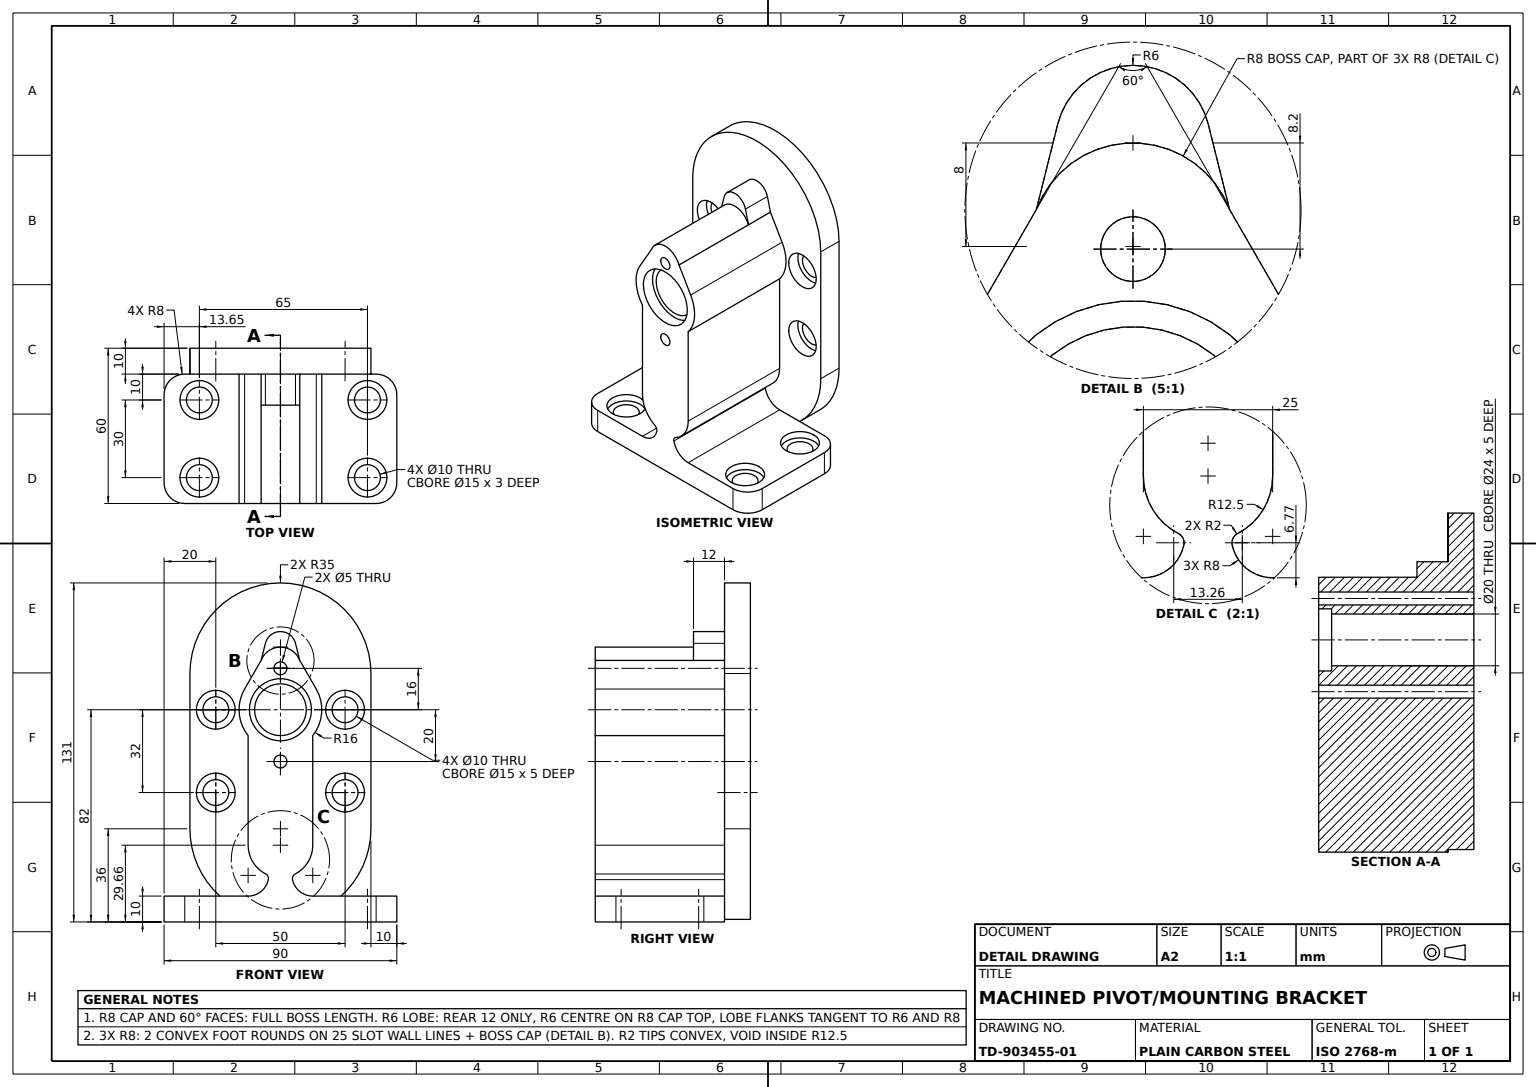
from build123d import *

# Parameters (mm, degrees)
FLANGE_PLATE_SKETCH_R     = 5
FLANGE_PLATE_DEPTH        = 10
FLANGE_START              = -5
FLANGE_RECESS_SKETCH_R    = 7.5
FLANGE_RECESS_SKETCH_R_2  = 5
FLANGE_RECESS_5MM_DEPTH   = 5
BRACKET_BODY_SKETCH_R     = 2.5
BRACKET_BODY_DEPTH        = 50
THROUGH_START             = -50
THROUGH_BORE_SKETCH_R     = 10
THROUGH_BORE_DEPTH        = 50
BORE_COUNTERBORE_SKETCH_R = 12
BORE_COUNTERBORE_24_DEPTH = 5
BODY_POCKET_SKETCH_R      = 5
BODY_POCKET_20MM_DEPTH    = 20
POCKET_STEP_SKETCH_R      = 7.5
POCKET_STEP_3MM_DEPTH     = 3
BODY_BOSS_12MM_DEPTH      = 12
BODY_FILLET_R8_A_R        = 8
BODY_FILLET_R8_B_R        = 8
BODY_SLOT_SKETCH_R        = 2.5
BODY_SLOT_CUT_DEPTH       = 112.126054551


with BuildPart() as part:
    # Flange Plate Sketch → Flange Plate (new body)
    with BuildSketch(Plane.XY):
        with BuildLine():
            Line((-35, -46), (-35, 14))
            ThreePointArc((-35, 14), (0, 49), (35, 14))
            Line((35, 14), (35, -46))
            ThreePointArc((35, -46), (0, -81), (-35, -46))
        make_face()
        with Locations((-25, 0)):
            Circle(FLANGE_PLATE_SKETCH_R, mode=Mode.SUBTRACT)
        with Locations((25, 0)):
            Circle(FLANGE_PLATE_SKETCH_R, mode=Mode.SUBTRACT)
        with Locations((-25, -32)):
            Circle(FLANGE_PLATE_SKETCH_R, mode=Mode.SUBTRACT)
        with Locations((25, -32)):
            Circle(FLANGE_PLATE_SKETCH_R, mode=Mode.SUBTRACT)
    extrude(amount=FLANGE_PLATE_DEPTH)

    # Flange Recess Sketch → Flange Recess 5mm (cut)
    # profile 1 of 4: a face of its own
    with BuildSketch(Plane.XY.offset(10).offset(FLANGE_START)):
        with Locations((-25, 0)):
            Circle(FLANGE_RECESS_SKETCH_R)
        with Locations((-25, 0)):
            Circle(FLANGE_RECESS_SKETCH_R_2, mode=Mode.SUBTRACT)
    # profile 2 of 4: a face of its own
    with BuildSketch(Plane.XY.offset(10).offset(FLANGE_START)):
        with Locations((25, 0)):
            Circle(FLANGE_RECESS_SKETCH_R)
        with Locations((25, 0)):
            Circle(FLANGE_RECESS_SKETCH_R_2, mode=Mode.SUBTRACT)
    # profile 3 of 4: a face of its own
    with BuildSketch(Plane.XY.offset(10).offset(FLANGE_START)):
        with Locations((25, -32)):
            Circle(FLANGE_RECESS_SKETCH_R)
        with Locations((25, -32)):
            Circle(FLANGE_RECESS_SKETCH_R_2, mode=Mode.SUBTRACT)
    # profile 4 of 4: a face of its own
    with BuildSketch(Plane.XY.offset(10).offset(FLANGE_START)):
        with Locations((-25, -32)):
            Circle(FLANGE_RECESS_SKETCH_R)
        with Locations((-25, -32)):
            Circle(FLANGE_RECESS_SKETCH_R_2, mode=Mode.SUBTRACT)
    extrude(amount=FLANGE_RECESS_5MM_DEPTH, mode=Mode.SUBTRACT)

    # Bracket Body Sketch → Bracket Body (add)
    # profile 1 of 2: a face of its own
    with BuildSketch(Plane.XY.offset(10)):
        with BuildLine():
            Line((-12.5, -72), (-23.430749028, -72))
            ThreePointArc((-23.430749028, -72), (0, -81), (23.430749028, -72))
            Line((23.430749028, -72), (12.5, -72))
            ThreePointArc((12.5, -72), (7.458524391, -70.211563707), (4.67113827, -65.645880922))
            ThreePointArc((4.67113827, -65.645880922), (4.822624016, -64.374561693), (5.714098019, -63.455608694))
            ThreePointArc((5.714098019, -63.455608694), (10.669494488, -58.85053718), (12.5, -52.33809621))
            Line((12.5, -52.33809621), (12.5, -9.987492178))
            ThreePointArc((12.5, -9.987492178), (15.954701786, -1.203117164), (13.856406461, 8))
            Line((13.856406461, 8), (7.473378872, 19.05572809))
            ThreePointArc((7.473378872, 19.05572809), (0, 24.201151372), (-7.473378872, 19.05572809))
            Line((-7.473378872, 19.05572809), (-13.856406461, 8))
            ThreePointArc((-13.856406461, 8), (-15.954701786, -1.203117164), (-12.5, -9.987492178))
            Line((-12.5, -9.987492178), (-12.5, -52.33809621))
            ThreePointArc((-12.5, -52.33809621), (-10.669494488, -58.85053718), (-5.714098019, -63.455608694))
            ThreePointArc((-5.714098019, -63.455608694), (-4.822624016, -64.374561693), (-4.67113827, -65.645880922))
            ThreePointArc((-4.67113827, -65.645880922), (-7.458524391, -70.211563707), (-12.5, -72))
        make_face()
        with Locations((0, -20)):
            Circle(BRACKET_BODY_SKETCH_R, mode=Mode.SUBTRACT)
        with BuildLine():
            ThreePointArc((0, -10), (-7.071067812, 7.071067812), (10, 0))
            ThreePointArc((10, 0), (7.071067812, -7.071067812), (0, -10))
        make_face(mode=Mode.SUBTRACT)
        with Locations((0, 16)):
            Circle(BRACKET_BODY_SKETCH_R, mode=Mode.SUBTRACT)
    # profile 2 of 2: a face of its own
    with BuildSketch(Plane.XY.offset(10)):
        with BuildLine():
            Line((-45, -72), (-45, -82))
            Line((-45, -82), (45, -82))
            Line((45, -82), (45, -72))
            Line((45, -72), (23.430749028, -72))
            ThreePointArc((23.430749028, -72), (0, -81), (-23.430749028, -72))
            Line((-23.430749028, -72), (-45, -72))
        make_face()
    extrude(amount=BRACKET_BODY_DEPTH)

    # Through Bore Sketch → Through Bore (cut)
    with BuildSketch(Plane.XY.offset(10).offset(THROUGH_START)):
        with Locations(Location((0, 0, 0), (0, 0, 180))):
            Circle(THROUGH_BORE_SKETCH_R)
    extrude(amount=THROUGH_BORE_DEPTH, mode=Mode.SUBTRACT)

    # Bore Counterbore Sketch → Bore Counterbore Ø24 (cut)
    with BuildSketch(Plane.XY.offset(60)):
        Circle(BORE_COUNTERBORE_SKETCH_R)
    extrude(amount=-BORE_COUNTERBORE_24_DEPTH, mode=Mode.SUBTRACT)

    # Body Pocket Sketch → Body Pocket 20mm (cut)
    with BuildSketch(Plane(origin=(0, -72, 0), x_dir=(1, 0, 0), z_dir=(0, 1, 0))):
        with Locations(Location((-31.350256263, -20, 0), (0, 0, 270))):
            Circle(BODY_POCKET_SKETCH_R)
        with Locations(Location((-31.350256263, -50, 0), (0, 0, 270))):
            Circle(BODY_POCKET_SKETCH_R)
        with Locations(Location((33.649743737, -20, 0), (0, 0, 270))):
            Circle(BODY_POCKET_SKETCH_R)
        with Locations(Location((33.649743737, -50, 0), (0, 0, 270))):
            Circle(BODY_POCKET_SKETCH_R)
    extrude(amount=-BODY_POCKET_20MM_DEPTH, mode=Mode.SUBTRACT)

    # Pocket Step Sketch → Pocket Step 3mm (cut)
    with BuildSketch(Plane(origin=(0, -72, 0), x_dir=(1, 0, 0), z_dir=(0, 1, 0))):
        with Locations(Location((-31.350256263, -20, 0), (0, 0, 270))):
            Circle(POCKET_STEP_SKETCH_R)
        with Locations(Location((-31.350256263, -50, 0), (0, 0, 270))):
            Circle(POCKET_STEP_SKETCH_R)
        with Locations(Location((33.649743737, -20, 0), (0, 0, 270))):
            Circle(POCKET_STEP_SKETCH_R)
        with Locations(Location((33.649743737, -50, 0), (0, 0, 270))):
            Circle(POCKET_STEP_SKETCH_R)
    extrude(amount=-POCKET_STEP_3MM_DEPTH, mode=Mode.SUBTRACT)

    # Body Boss Sketch → Body Boss 12mm (add)
    with BuildSketch(Plane.XY.offset(10)):
        with BuildLine():
            Line((7.473378872, 19.05572809), (5.820364134, 25.658327183))
            ThreePointArc((5.820364134, 25.658327183), (0, 30.201151372), (-5.820364134, 25.658327183))
            Line((-5.820364134, 25.658327183), (-7.473378872, 19.05572809))
            ThreePointArc((-7.473378872, 19.05572809), (0, 24.201151372), (7.473378872, 19.05572809))
        make_face()
    extrude(amount=BODY_BOSS_12MM_DEPTH)

    # Body Fillet R8 A
    body_fillet_r8_a_edges = [part.edges().sort_by_distance(p)[0] for p in [
        (-45, -77, 60),
        (45, -77, 60),
    ]]
    fillet(body_fillet_r8_a_edges, radius=BODY_FILLET_R8_A_R)

    # Body Fillet R8 B
    body_fillet_r8_b_edges = [part.edges().sort_by_distance(p)[0] for p in [
        (-45, -77, 10),
        (45, -77, 10),
    ]]
    fillet(body_fillet_r8_b_edges, radius=BODY_FILLET_R8_B_R)

    # Body Slot Sketch → Body Slot Cut (cut, through all)
    with BuildSketch(Plane.XY.offset(60)):
        with Locations((0, 16)):
            Circle(BODY_SLOT_SKETCH_R)
        with Locations((0, -20)):
            Circle(BODY_SLOT_SKETCH_R)
    extrude(amount=-BODY_SLOT_CUT_DEPTH, mode=Mode.SUBTRACT)


solid = part.part
